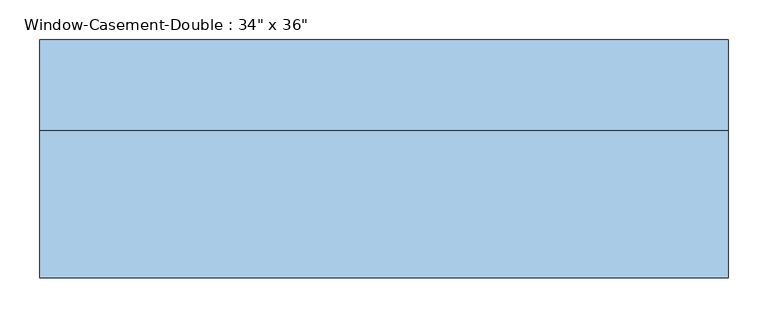
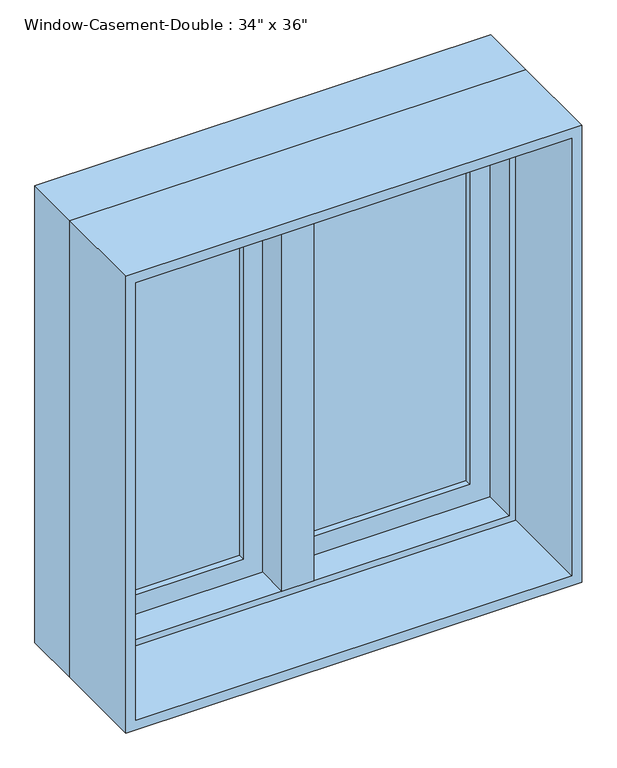
"""IFC4 building model written with IfcOpenShell, lengths in millimetres: window geometry."""

from ifc_helpers import new_model, si_unit, frame, origin, place, context, project, spatial, polyline, outline, extrude, faceted_brep, source, transform, mapped, element, save


def window_6eb120d7(model_context):
    return source(origin(), model_context, "Body", "SolidModel", [
        faceted_brep([(9.525, 158.75, 1816.1), (-9.525, 158.75, 1816.1), (-9.525, 107.95, 1816.1), (9.525, 107.95, 1816.1), (9.525, 158.75, 927.1), (9.525, 107.95, 927.1), (-9.525, 107.95, 927.1), (-9.525, 158.75, 927.1), (-9.525, 107.95, 946.15), (-9.525, 107.95, 1797.05), (-30.1625, 107.95, 946.15), (-30.1625, 107.95, 1797.05), (-30.1625, 44.45, 946.15), (-30.1625, 44.45, 1797.05), (30.1625, 44.45, 946.15), (30.1625, 44.45, 1797.05), (30.1625, 107.95, 946.15), (30.1625, 107.95, 1797.05), (9.525, 107.95, 946.15), (9.525, 107.95, 1797.05)], [[[0, 1, 2, 3]], [[4, 5, 6, 7]], [[1, 0, 4, 7]], [[2, 1, 7, 6, 8, 9]], [[9, 8, 10, 11]], [[11, 10, 12, 13]], [[13, 12, 14, 15]], [[15, 14, 16, 17]], [[17, 16, 18, 19]], [[0, 3, 19, 18, 5, 4]], [[18, 8, 6, 5]], [[9, 19, 3, 2]], [[8, 18, 16, 14, 12, 10]], [[19, 9, 11, 13, 15, 17]]]),
        extrude(outline(polyline([(-66.675, 139.7), (-66.675, 133.35), (-361.95, 133.35), (-361.95, 139.7), (-66.675, 139.7)])), frame((0.0, 0.0, 984.25), z_axis=(0.0, 0.0, 1.0), x_axis=(1.0, 0.0, 0.0)), (0.0, 0.0, 1.0), 774.7),
        extrude(outline(polyline([(-361.95, 120.65), (-361.95, 127.0), (-66.675, 127.0), (-66.675, 120.65), (-361.95, 120.65)])), frame((0.0, 0.0, 984.25), z_axis=(0.0, 0.0, 1.0), x_axis=(1.0, 0.0, 0.0)), (0.0, 0.0, 1.0), 774.7),
        extrude(outline(polyline([(361.95, 139.7), (361.95, 133.35), (66.675, 133.35), (66.675, 139.7), (361.95, 139.7)])), frame((0.0, 0.0, 984.25), z_axis=(0.0, 0.0, 1.0), x_axis=(1.0, 0.0, 0.0)), (0.0, 0.0, 1.0), 774.7),
        extrude(outline(polyline([(66.675, 120.65), (66.675, 127.0), (361.95, 127.0), (361.95, 120.65), (66.675, 120.65)])), frame((0.0, 0.0, 984.25), z_axis=(0.0, 0.0, 1.0), x_axis=(1.0, 0.0, 0.0)), (0.0, 0.0, 1.0), 774.7),
        extrude(outline(polyline([(1816.1, -419.1), (927.1, -419.1), (927.1, -9.525), (1816.1, -9.525), (1816.1, -419.1)]), holes=[polyline([(1758.95, -66.675), (984.25, -66.675), (984.25, -361.95), (1758.95, -361.95), (1758.95, -66.675)])]), frame((0.0, 107.95, 0.0), z_axis=(0.0, 1.0, 0.0), x_axis=(0.0, 0.0, 1.0)), (0.0, 0.0, 1.0), 44.45),
        extrude(outline(polyline([(927.1, 419.1), (1816.1, 419.1), (1816.1, 9.525), (927.1, 9.525), (927.1, 419.1)]), holes=[polyline([(984.25, 66.675), (1758.95, 66.675), (1758.95, 361.95), (984.25, 361.95), (984.25, 66.675)])]), frame((0.0, 107.95, 0.0), z_axis=(0.0, 1.0, 0.0), x_axis=(0.0, 0.0, 1.0)), (0.0, 0.0, 1.0), 44.45),
        extrude(outline(polyline([(1828.8, -431.8), (914.4, -431.8), (914.4, 431.8), (1828.8, 431.8), (1828.8, -431.8)]), holes=[polyline([(1809.75, 412.75), (933.45, 412.75), (933.45, -412.75), (1809.75, -412.75), (1809.75, 412.75)])]), frame((0.0, -139.7, 0.0), z_axis=(0.0, 1.0, 0.0), x_axis=(0.0, 0.0, 1.0)), (0.0, 0.0, 1.0), 184.15),
        faceted_brep([(400.05, 107.95, 1797.05), (400.05, 44.45, 1797.05), (-400.05, 44.45, 1797.05), (-400.05, 107.95, 1797.05), (419.1, 158.75, 1816.1), (419.1, 107.95, 1816.1), (-419.1, 107.95, 1816.1), (-419.1, 158.75, 1816.1), (431.8, 44.45, 1828.8), (431.8, 158.75, 1828.8), (-431.8, 158.75, 1828.8), (-431.8, 44.45, 1828.8), (-400.05, 44.45, 946.15), (-400.05, 107.95, 946.15), (-419.1, 107.95, 927.1), (-419.1, 158.75, 927.1), (-431.8, 158.75, 914.4), (-431.8, 44.45, 914.4), (400.05, 44.45, 946.15), (400.05, 107.95, 946.15), (419.1, 107.95, 927.1), (419.1, 158.75, 927.1), (431.8, 158.75, 914.4), (431.8, 44.45, 914.4)], [[[0, 1, 2, 3]], [[4, 5, 6, 7]], [[8, 9, 10, 11]], [[3, 2, 12, 13]], [[7, 6, 14, 15]], [[11, 10, 16, 17]], [[13, 12, 18, 19]], [[15, 14, 20, 21]], [[17, 16, 22, 23]], [[11, 17, 23, 8], [1, 18, 12, 2]], [[19, 18, 1, 0]], [[5, 20, 14, 6], [3, 13, 19, 0]], [[21, 20, 5, 4]], [[23, 22, 9, 8]], [[9, 22, 16, 10], [7, 15, 21, 4]]]),
    ])


if __name__ == "__main__":
    model = new_model("IFC4")
    model_context = context("Model", 3, world=origin())
    ifc_project = project(units=[si_unit("LENGTHUNIT", "METRE", prefix="MILLI")], contexts=[model_context])
    site = spatial("IfcSite", under=ifc_project)
    building = spatial("IfcBuilding", under=site)
    placement = place(None, origin())
    window_shape = window_6eb120d7(model_context)
    element("IfcWindow", 1, ObjectType="Window-Casement-Double : 34\" x 36\"", at=placement, inside=building, context=model_context, shape_type="MappedRepresentation", body=[
        mapped(window_shape, transform((0.0, 0.0, 0.0), x_axis=(1.0, 0.0, 0.0), y_axis=(0.0, 1.0, 0.0), z_axis=(0.0, 0.0, 1.0))),
    ])
    save(model, "model.ifc")

# Revit data of these elements
# Type "Window-Casement-Double : 34\" x 36\""
#   Type Mark = "14"
#   Fire Rating = "0.5h"
#   Assembly Code = "B2020100"
#   Analytic Construction = "Double glazing - domestic"
#   Frame Extension [instance default] = 0' - 0 1/4"
#   Window Inset [instance default] = 0' - 0"
#   Wall Thickness [instance default] = 0' - 6"
#   Interior Wall Closure [instance default] = 0' - 2 1/4"
#   Half Width = 1' - 5"
#   Visual Light Transmittance = 0.81
#   Thermal Resistance (R) = 1.8146 (h·ft²·°F)/BTU
#   Solar Heat Gain Coefficient = 0.76
#   Rough Width = 2' - 10 1/2"
#   Rough Height = 3' - 0 1/2"
#   Height = 3' - 0"
#   Heat Transfer Coefficient (U) = 0.5511 BTU/(h·ft²·°F)
#   Exterior Wall Closure [instance default] = 0' - 1 1/4"
#   Extension Jamb [instance default] = 0' - 2 1/4"
#   Default Sill Height = 3' - 0"
#   Width = 2' - 10"
#   Define Thermal Properties by = 0
#   Muntin Visibility = yes
#   Interior Trim Visibility [instance default] = yes
#   Exterior Trim Visibility [instance default] = yes
#   Extension Jamb Visibility [instance default] = yes
#   Interior Trim Material = Wood - Stained
#   Muntin Pattern = Muntin Pattern_2x2 : Muntin Pattern_2x2
#   Interior Trim = Trim-Window-Interior-Flat : Picture Frame
#   Interior Frame Material = Wood - Stained
#   Glass Panel Material = Glass
#   Exterior Trim Material = Clad - White
#   Exterior Trim = Trim-Window-Exterior-Flat : with Sill
#   Exterior Frame Material = Clad - White
#   Wall Closure = (empty or 0)
# Element 1 (IfcWindow, "Window-Casement-Double : 34\" x 36\"")
#   Wall Thickness = 0' - 11"
#   Extension Jamb = 0' - 7 1/4"
#   Materials on its faces: "Wood - Stained", "Glass", "Clad - White"
# Materials
#   "Wood - Stained": class "Wood", colour RGB 224 178 126, transparency 0, Cost = 0
#   "Glass": class "Glass", colour RGB 0 128 192, transparency 0.75, Description = "Soda Lime Glass", Cost = 0
#   "Clad - White": class "Wood", colour RGB 242 242 238, transparency 0, Cost = 0
